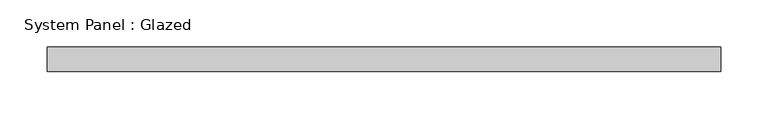
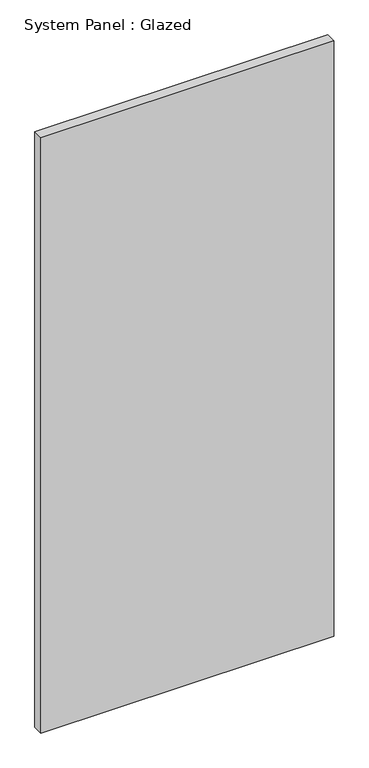
"""IFC4 building model written with IfcOpenShell, lengths in millimetres: plate geometry, System Panel : Glazed."""

from ifc_helpers import new_model, si_unit, origin, origin_with_axes, place, context, project, spatial, polyline, outline, extrude, source, transform, mapped, element, save


def system_panel_glazed_b3daaad5(model_context):
    return source(origin(), model_context, "Body", "SweptSolid", [
        extrude(outline(polyline([(354.2306477, 19.05), (-354.2306477, 19.05), (-354.2306477, 44.45), (354.2306477, 44.45), (354.2306477, 19.05)])), origin_with_axes(), (0.0, 0.0, 1.0), 1522.9537661),
    ])


if __name__ == "__main__":
    model = new_model("IFC4")
    model_context = context("Model", 3, world=origin())
    ifc_project = project(units=[si_unit("LENGTHUNIT", "METRE", prefix="MILLI")], contexts=[model_context])
    site = spatial("IfcSite", under=ifc_project)
    building = spatial("IfcBuilding", under=site)
    placement = place(None, origin())
    system_panel_glazed_shape = system_panel_glazed_b3daaad5(model_context)
    element("IfcPlate", 1, ObjectType="System Panel : Glazed", at=placement, inside=building, context=model_context, shape_type="MappedRepresentation", body=[
        mapped(system_panel_glazed_shape, transform((0.0, 0.0, 0.0), x_axis=(1.0, 0.0, 0.0), y_axis=(0.0, 1.0, 0.0), z_axis=(0.0, 0.0, 1.0))),
    ])
    save(model, "model.ifc")

# Revit data of these elements
# Type "System Panel : Glazed"
#   Construction Type Id = "GSP4R"
#   Analytic Construction = "1/8 in Pilkington single glazing"
#   Visual Light Transmittance = 0.9
#   Solar Heat Gain Coefficient = 0.86
#   Heat Transfer Coefficient (U) = 1.18115 BTU/(h·ft²·°F)
#   Define Thermal Properties by = 1
# Element 1 (IfcPlate, "System Panel : Glazed")
#   Materials on its faces: "Glass"
# Materials
#   "Glass": class "Glass", colour RGB 0 128 192, transparency 0.75, Description = "Soda Lime Glass", Cost = 0
